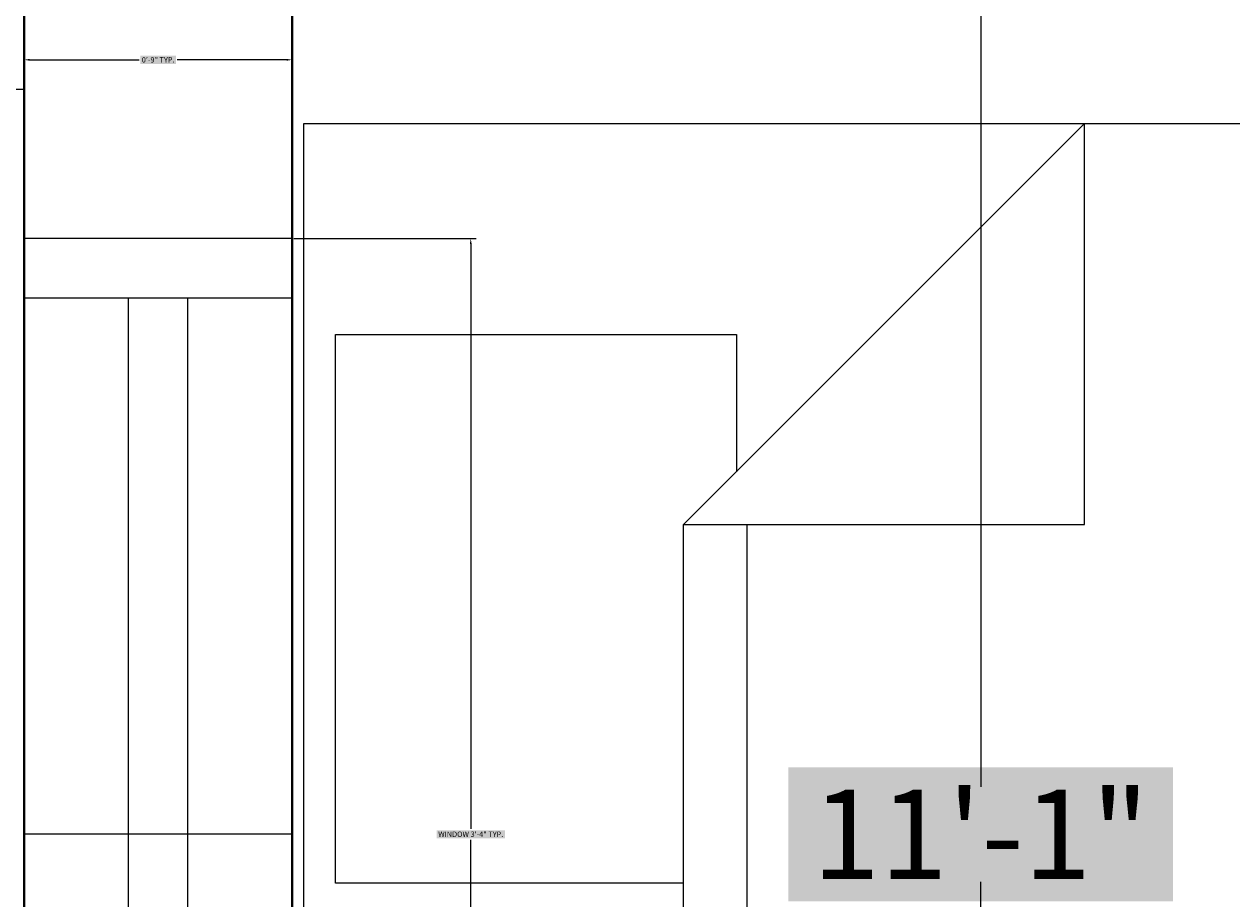
# Model space of a CAD drawing. Units: inches. Extents: x -301 to 715, y -607 to 364.
# Tile 72 of 141: x -205 to -164, y -3 to 26. Entities that reach past the tile are written whole.
import ezdxf

# ---------------------------------------------------------------- set-up
doc = ezdxf.new("R2010")
doc.units = ezdxf.units.IN
doc.header["$MEASUREMENT"] = 0
doc.linetypes.add('ACAD_ISO02W100', pattern=[15, 12, -3])
for name, color, linetype, lineweight in [('A-ANNO-DIMS', 2, 'Continuous', 18), ('A-FURN', 8, 'Continuous', 18), ('A-GLAZ', 2, 'Continuous', 25), ('A-GLAZ-OVHD', 2, 'ACAD_ISO02W100', 18), ('A-WALL', 3, 'Continuous', 40)]:
    doc.layers.add(name, color=color, linetype=linetype, lineweight=lineweight)
doc.styles.get("Standard").update_dxf_attribs({"font": 'arial.ttf'})
doc.dimstyles.get("Standard").update_dxf_attribs({"dimtxt": 0.18, "dimasz": 0.18, "dimexe": 0.18, "dimexo": 0.0625, "dimgap": 0.09, "dimtad": 0, "dimtih": 1, "dimtoh": 1, "dimdec": 1, "dimzin": 0, "dimdsep": 46, "dimlunit": 4, "dimtxsty": 'Standard', "dimcen": 0.09, "dimclrd": 3, "dimclre": 4, "dimclrt": 6, "dimadec": 0, "dimazin": 0, "dimtfac": 1, "dimtdec": 1, "dimtofl": 0, "dimtmove": 0, "dimatfit": 3, "dimfxl": 1, "dimtfill": 2, "dimtfillclr": 51, "dimtolj": 1, "dimtzin": 0, "dimarcsym": 0})

# ---------------------------------------------------------------- blocks, each defined once
blk = doc.blocks.new('Bed - Queen')
for p, q in [((0, 0), (59.99999, 0)), ((59.99999, 0), (59.99999, -80.00003)), ((31.19999, -1.2), (51.99999, -1.2)), ((31.19999, -14.4), (31.19999, -1.2)), ((51.99999, -1.2), (51.99999, -16.4)), ((0, -14.4), (44.8, -14.4)), ((59.99999, -29.6), (44.8, -14.4)), ((44.8, -14.4), (44.8, -29.6)), ((51.99999, -16.4), (46.79936, -16.4)), ((44.8, -16.8), (0, -16.8)), ((44.8, -29.6), (59.99999, -29.6))]:
    blk.add_line(p, q)
blk = doc.blocks.new('*D56')
at = {"layer": 'A-ANNO-DIMS', "color": 0, "lineweight": -2, "transparency": 16777216}
for p, q in [((-195.541, 65.682), (-172.295, 65.682)), ((-172.475, 60.682), (-172.475, 0.778)), ((-172.475, -62.318), (-172.475, -2.414)), ((-195.541, -67.318), (-172.295, -67.318))]:
    blk.add_line(p, q, dxfattribs=at)
at = {"layer": 'A-ANNO-DIMS', "color": 0, "transparency": 16777216}
for points in [[(-173.308, 60.682), (-171.641, 60.682), (-172.475, 65.682)], [(-173.308, -62.318), (-171.641, -62.318), (-172.475, -67.318)]]:
    blk.add_solid(points, dxfattribs=at)
at = {"layer": 'Defpoints', "color": 0, "transparency": 16777216}
for p in [(-195.603, 65.682), (-172.475, 65.682), (-195.603, -67.318)]:
    blk.add_point(p, dxfattribs=at)
at = {"layer": 'A-ANNO-DIMS', "color": 0, "transparency": 16777216, "insert": (-172.475, -0.818), "char_height": 3, "attachment_point": 5, "bg_fill": 1, "box_fill_scale": 1.25, "bg_fill_color": 51, "bg_fill_transparency": 0}
blk.add_mtext('\\A1;11\'-1"', dxfattribs=at)
blk = doc.blocks.new('WIN-36-PLAN')
for p, q in [((20, 0), (20, 9)), ((38, 0), (38, 9)), ((40, 0), (40, 9)), ((2, 5.5), (38, 5.5)), ((2, 3.5), (38, 3.5))]:
    blk.add_line(p, q)
blk = doc.blocks.new('WIN-SHADE-50')
at = {"ltscale": 1.5}
for p, q in [((50, 0), (50, 12)), ((45, 0), (50, 0))]:
    blk.add_line(p, q, dxfattribs=at)
blk = doc.blocks.new('*D96')
at = {"layer": 'A-ANNO-DIMS', "color": 4, "lineweight": -2, "transparency": 16777216}
for p, q in [((-195.541, 19.182), (-189.423, 19.182)), ((-195.541, -20.818), (-189.423, -20.818))]:
    blk.add_line(p, q, dxfattribs=at)
at = {"layer": 'A-ANNO-DIMS', "color": 3, "lineweight": -2, "transparency": 16777216}
for p, q in [((-189.603, 19.002), (-189.603, -0.634)), ((-189.603, -20.638), (-189.603, -1.001))]:
    blk.add_line(p, q, dxfattribs=at)
at = {"layer": 'A-ANNO-DIMS', "color": 3, "transparency": 16777216}
for points in [[(-189.633, 19.002), (-189.573, 19.002), (-189.603, 19.182)], [(-189.633, -20.638), (-189.573, -20.638), (-189.603, -20.818)]]:
    blk.add_solid(points, dxfattribs=at)
at = {"layer": 'Defpoints', "color": 0, "transparency": 16777216}
for p in [(-195.603, 19.182), (-189.603, 19.182), (-195.603, -20.818)]:
    blk.add_point(p, dxfattribs=at)
at = {"layer": 'A-ANNO-DIMS', "color": 6, "transparency": 16777216, "insert": (-189.603, -0.818), "char_height": 0.18, "attachment_point": 5, "bg_fill": 1, "box_fill_scale": 1.25, "bg_fill_color": 51, "bg_fill_transparency": 0}
blk.add_mtext('\\A1;WINDOW 3\'-4" TYP.', dxfattribs=at)
blk = doc.blocks.new('*D97')
at = {"layer": 'A-ANNO-DIMS', "color": 4, "lineweight": -2, "transparency": 16777216}
for p, q in [((-204.603, 19.245), (-204.603, 25.362)), ((-195.603, 19.245), (-195.603, 25.362))]:
    blk.add_line(p, q, dxfattribs=at)
at = {"layer": 'A-ANNO-DIMS', "color": 3, "lineweight": -2, "transparency": 16777216}
for p, q in [((-204.423, 25.182), (-200.742, 25.182)), ((-195.783, 25.182), (-199.465, 25.182))]:
    blk.add_line(p, q, dxfattribs=at)
at = {"layer": 'A-ANNO-DIMS', "color": 3, "transparency": 16777216}
for points in [[(-204.423, 25.212), (-204.423, 25.152), (-204.603, 25.182)], [(-195.783, 25.212), (-195.783, 25.152), (-195.603, 25.182)]]:
    blk.add_solid(points, dxfattribs=at)
at = {"layer": 'Defpoints', "color": 0, "transparency": 16777216}
for p in [(-204.603, 25.182), (-204.603, 19.182), (-195.603, 19.182)]:
    blk.add_point(p, dxfattribs=at)
at = {"layer": 'A-ANNO-DIMS', "color": 6, "transparency": 16777216, "insert": (-200.103, 25.182), "char_height": 0.18, "attachment_point": 5, "bg_fill": 1, "box_fill_scale": 1.25, "bg_fill_color": 51, "bg_fill_transparency": 0}
blk.add_mtext('\\A1;0\'-9" TYP.', dxfattribs=at)
blk = doc.blocks.new('*D151')
at = {"layer": 'A-ANNO-DIMS', "color": 4, "lineweight": -2, "transparency": 16777216}
for p, q in [((-204.603, -223.755), (-204.603, 359.612)), ((-45.603, -214.755), (-45.603, 359.612))]:
    blk.add_line(p, q, dxfattribs=at)
at = {"layer": 'A-ANNO-DIMS', "color": 3, "lineweight": -2, "transparency": 16777216}
for p, q in [((-204.423, 359.432), (-125.494, 359.432)), ((-45.783, 359.432), (-124.713, 359.432))]:
    blk.add_line(p, q, dxfattribs=at)
at = {"layer": 'A-ANNO-DIMS', "color": 3, "transparency": 16777216}
for points in [[(-204.423, 359.462), (-204.423, 359.402), (-204.603, 359.432)], [(-45.783, 359.462), (-45.783, 359.402), (-45.603, 359.432)]]:
    blk.add_solid(points, dxfattribs=at)
at = {"layer": 'Defpoints', "color": 0, "transparency": 16777216}
for p in [(-45.603, 359.432), (-45.603, -214.818), (-204.603, -223.818)]:
    blk.add_point(p, dxfattribs=at)
at = {"layer": 'A-ANNO-DIMS', "color": 6, "transparency": 16777216, "insert": (-125.103, 359.432), "char_height": 0.18, "attachment_point": 5, "bg_fill": 1, "box_fill_scale": 1.25, "bg_fill_color": 51, "bg_fill_transparency": 0}
blk.add_mtext('\\A1;13\'-3"', dxfattribs=at)

msp = doc.modelspace()

# ---------------------------------------------------------------- linework, layer by layer
at = {"layer": 'A-WALL'}
for p, q in [((-204.603, 71.682), (-204.603, -67.318)), ((-195.603, 65.682), (-195.603, -67.318))]:
    msp.add_line(p, q, dxfattribs=at)

# ---------------------------------------------------------------- block references
at = {"layer": 'A-FURN', "xscale": 0.8856750462000775, "yscale": 0.8856750462000775, "zscale": 0.8856750462000775, "rotation": 90}
msp.add_blockref('Bed - Queen', (-195.207, -30.095), dxfattribs=at)
at = {"layer": 'A-GLAZ', "rotation": 90.00000000000043}
msp.add_blockref('WIN-36-PLAN', (-195.603, -20.817), dxfattribs=at)
at = {"layer": 'A-GLAZ-OVHD', "rotation": 90.00000000000011}
msp.add_blockref('WIN-SHADE-50', (-204.603, -25.817), dxfattribs=at)

# ---------------------------------------------------------------- dimensions: what is measured, and where the dimension line sits
at = {"layer": 'A-ANNO-DIMS'}
dim = msp.add_linear_dim(base=(-45.603, 359.432), p1=(-204.603, -223.818), p2=(-45.603, -214.818), dimstyle='Standard', override={"dimdec": 1, "dimlfac": 1, "dimrnd": 0, "dimzin": 1, "dimdsep": 46, "dimlunit": 4, "dimfrac": 2}, dxfattribs=at)
dim.commit()
dim.dimension.update_dxf_attribs({"geometry": '*D151', "text_midpoint": (-125.103, 359.432)})
dim = msp.add_linear_dim(base=(-172.475, 65.682), p1=(-195.603, -67.318), p2=(-195.603, 65.682), angle=90, dimstyle='Standard', override={"dimtxt": 3, "dimasz": 5, "dimclrd": 0, "dimclre": 0, "dimclrt": 0}, dxfattribs=at)
dim.commit()
dim.dimension.update_dxf_attribs({"geometry": '*D56', "text_midpoint": (-172.475, -0.818)})
for base, p1, p2, angle, text, picture, middle in [((-204.603, 25.182), (-195.603, 19.182), (-204.603, 19.182), 180, '<> TYP.', '*D97', (-200.103, 25.182)), ((-189.603, 19.182), (-195.603, -20.818), (-195.603, 19.182), 90, 'WINDOW <> TYP.', '*D96', (-189.603, -0.818))]:
    dim = msp.add_linear_dim(base=base, p1=p1, p2=p2, angle=angle, text=text, dimstyle='Standard', override={"dimdec": 1, "dimlfac": 1, "dimrnd": 0, "dimzin": 1, "dimdsep": 46, "dimlunit": 4, "dimfrac": 2}, dxfattribs=at)
    dim.commit()
    dim.dimension.update_dxf_attribs({"geometry": picture, "text_midpoint": middle})

doc.saveas('drawing.dxf')
